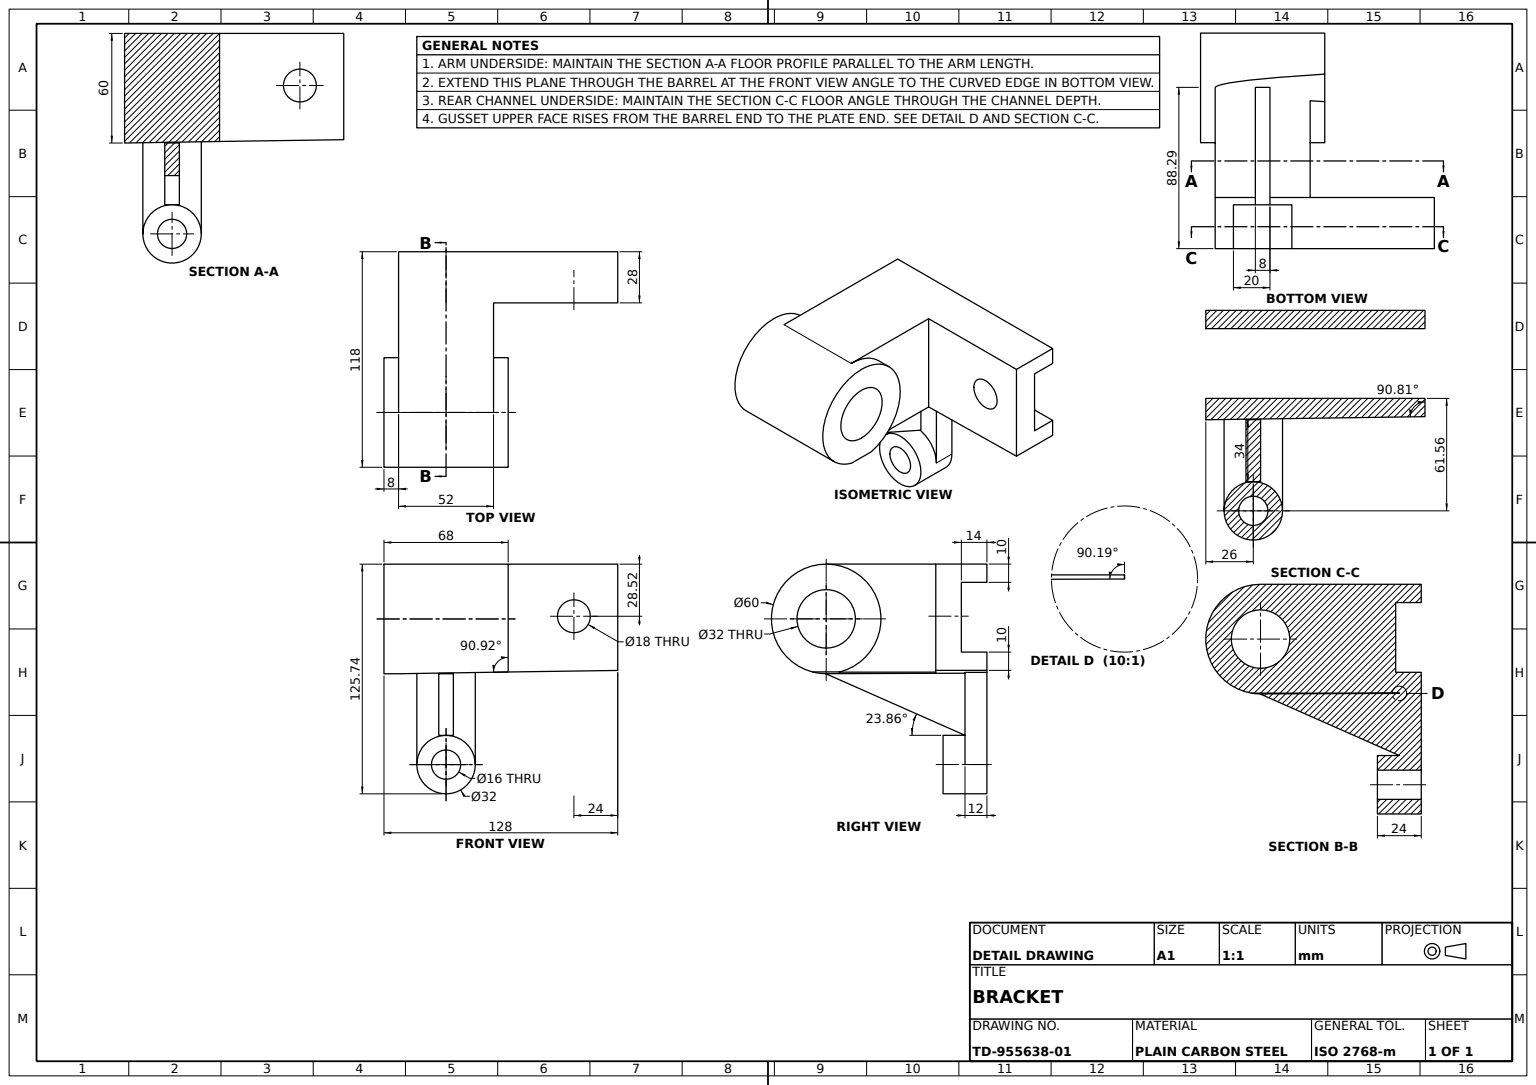
SolidWorks part; units mm, degrees
material "Plain Carbon Steel"
ref_plane "Front Plane" through (0, 0, 0) normal (0, 0, 1) x (1, 0, 0)
ref_plane "Top Plane" through (0, 0, 0) normal (0, 1, 0) x (1, 0, 0)
ref_plane "Right Plane" through (0, 0, 0) normal (1, 0, 0) x (0, 0, -1)
sketch "Base Block Sketch" plane through (0, 0, 0) normal (0, 0, 1) x (1, 0, 0)
  line L0 (0, 0) -> (128, 1.8156)
  line L1 (128, 1.8156) -> (128, 60)
  line L2 (128, 60) -> (0, 60)
  line L3 (0, 60) -> (0, 0)
  dimension "D1" = 128
  dimension "D2" = 60
  dimension "D3" = 0.813
extrude "Base Block" add sketch "Base Block Sketch" along normal blind 28
sketch "Upright Wall Sketch" plane through (0, 0, 0) normal (-1, 0, 0) x (0, 0, 1)
  line L0 (88, 60) -> (88, 0)
  line L3 (88, 0) -> (28, 0)
  line L4 (28, 0) -> (28, 60)
  line L5 (28, 60) -> (88, 60)
  dimension "D1" = 60
extrude "Upright Wall" add sketch "Upright Wall Sketch" against normal blind 68
sketch "Bearing Boss Sketch" plane through (68, 0, 0) normal (1, 0, 0) x (0, 0, -1)
  line L0 (-88, 0) -> (-88, 60) construction
  circle A0 centre (-88, 30) radius 30
  dimension "D1" = 60
  dimension "D2" = 60
extrude "Bearing Boss Ø60" add sketch "Bearing Boss Sketch" against normal blind 68
sketch "Bearing Bore Sketch" plane through (68, 0, 0) normal (1, 0, 0) x (0, 0, -1)
  circle A0 centre (-88, 30) radius 16
  dimension "D1" = 32
  dimension "D2" = 32
extrude "Bearing Bore Ø32" cut sketch "Bearing Bore Sketch" against normal blind 68
sketch "Base Profile Cut Sketch" plane through (128, 0, 0) normal (1, 0, 0) x (0, 0, -1)
  line L0 (0, 50) -> (-14, 50)
  line L1 (0, 1.8156) -> (0, 60) construction
  line L2 (0, 50) -> (0, 11.8156)
  line L3 (-28, 60) -> (0, 60) construction
  line L4 (-14, 30.9078) -> (-14, 11.8156)
  line L5 (-14, 11.8156) -> (0, 11.8156)
  line L7 (0, 50) -> (-14, 50)
  line L8 (-14, 50) -> (-14, 30.9078)
  line M1 (0, 1.8156) -> (0, 60)
  dimension "D1" = 14
  dimension "D2" = 10
  dimension "D3" = 29.0922
extrude "Base Profile Cut" cut sketch "Base Profile Cut Sketch" against normal blind 128 contours L0 L8 L4 L5 M1
sketch "Through Hole Sketch" plane through (0, 0, 28) normal (0, 0, 1) x (1, 0, 0)
  line L0 (128, 1.8156) -> (128, 60) construction
  line L1 (68, 0.9645) -> (128, 1.8156) construction
  circle A0 centre (104, 31.4782) radius 9
  dimension "D1" = 18
  dimension "D4" = 18
  dimension "D2" = 24
  dimension "D3" = 30
extrude "Through Hole Ø18" cut sketch "Through Hole Sketch" against normal blind 128
sketch "End Channel Recess Sketch" plane through (0, 0, 0) normal (-1, 0, 0) x (0, 0, 1)
  line L0 (0, 60) -> (88, 60)
  line L1 (0, 0) -> (88, 0)
  line L2 (0, 60) -> (0, 50)
  line L3 (0, 60) -> (0, 50) construction
  line L4 (0, 50) -> (14, 50) construction
  line L5 (0, 50) -> (14, 50)
  line L6 (14, 50) -> (14, 11.8156)
  line L7 (14, 11.8156) -> (0, 11.8156)
  line L8 (0, 11.8156) -> (0, 0)
  arc A0 (88, 60) -> (88, 0) centre (88, 30) ccw
  dimension "D1" = 60
extrude "End Channel Recess" cut sketch "End Channel Recess Sketch" against normal blind 8
sketch "Wall Recess Sketch" plane through (68, 0, 0) normal (1, 0, 0) x (0, 0, -1)
  line L0 (-28, 60) -> (-28, 0)
  line L1 (-28, 0) -> (-88, 0)
  line L3 (-88, 60) -> (-28, 60)
  arc A0 (-88, 0) -> (-88, 60) centre (-88, 30) ccw
  dimension "D1" = 60
extrude "Wall Recess" cut sketch "Wall Recess Sketch" against normal blind 8
sketch "Triangular Relief Sketch" plane through (0, 0, 28) normal (0, 0, -1) x (-1, 0, 0)
  line L0 (-68, 0) -> (-68, 0.9645)
  line L1 (-8, 0.1135) -> (-128, 1.8156) construction
  line L2 (-68, 0.9645) -> (-8, 0)
  line L3 (-8, 0) -> (-68, 0)
extrude "Triangular Relief Cut" cut sketch "Triangular Relief Sketch" against normal blind 100
sketch "Side Lug Plate Sketch" plane through (0, 0, 0) normal (0, 0, -1) x (-1, 0, 0)
  line L0 (-8, 11.8156) -> (-8, 0.1135) construction
  line L2 (-50, -49.7447) -> (-50, 0.7092)
  line L3 (-8, 0.1135) -> (-128, 1.8156) construction
  line L4 (-50, 0.7092) -> (-18, 0.2553)
  line L5 (-18, 0.2553) -> (-18, -49.7447)
  arc A1 (-50, -49.7447) -> (-18, -49.7447) centre (-34, -49.7447) ccw
  dimension "D1" = 16
  dimension "D2" = 32
  dimension "D3" = 26
  dimension "D4" = 61.5603
extrude "Side Lug Plate" add sketch "Side Lug Plate Sketch" against normal blind 12
sketch "Lug Boss Sketch" plane through (0, 0, 12) normal (0, 0, 1) x (1, 0, 0)
  circle A0 centre (34, -49.7447) radius 16
  dimension "D1" = 32
  dimension "D2" = 32
extrude "Lug Boss Ø32" add sketch "Lug Boss Sketch" along normal blind 12
sketch "Lug Gusset Sketch" plane through (50, 0, 0) normal (1, 0, 0) x (0, 0, -1)
  line L0 (-12, 0.2553) -> (-12, -33.7447)
  line L1 (-12, -33.7447) -> (-88.2925, 0)
  line L2 (-88.2925, 0) -> (-12, 0.2553)
  line L3 (0, 0.7092) -> (0, -49.7447) construction
  line L4 (-12, 0.7092) -> (0, 0.7092) construction
  dimension "D1" = 88.2925
  dimension "D2" = 0.7092
extrude "Lug Gusset" add sketch "Lug Gusset Sketch" against normal blind 20
sketch "Gusset Trim Sketch" plane through (50, 0, 0) normal (1, 0, 0) x (0, 0, -1)
  line L0 (-88.2925, 0) -> (-12, 0.2553)
  line L1 (-12, 0.2553) -> (-12, -33.7447)
  line L2 (-12, -33.7447) -> (-88.2925, 0)
extrude "Gusset Trim Cut" cut sketch "Gusset Trim Sketch" against normal blind 12
sketch "Lug Hole Sketch" plane through (0, 0, 24) normal (0, 0, 1) x (1, 0, 0)
  circle A0 centre (34, -49.7447) radius 8
  dimension "D1" = 16
  dimension "D2" = 16
extrude "Lug Hole Ø16" cut sketch "Lug Hole Sketch" against normal blind 24
